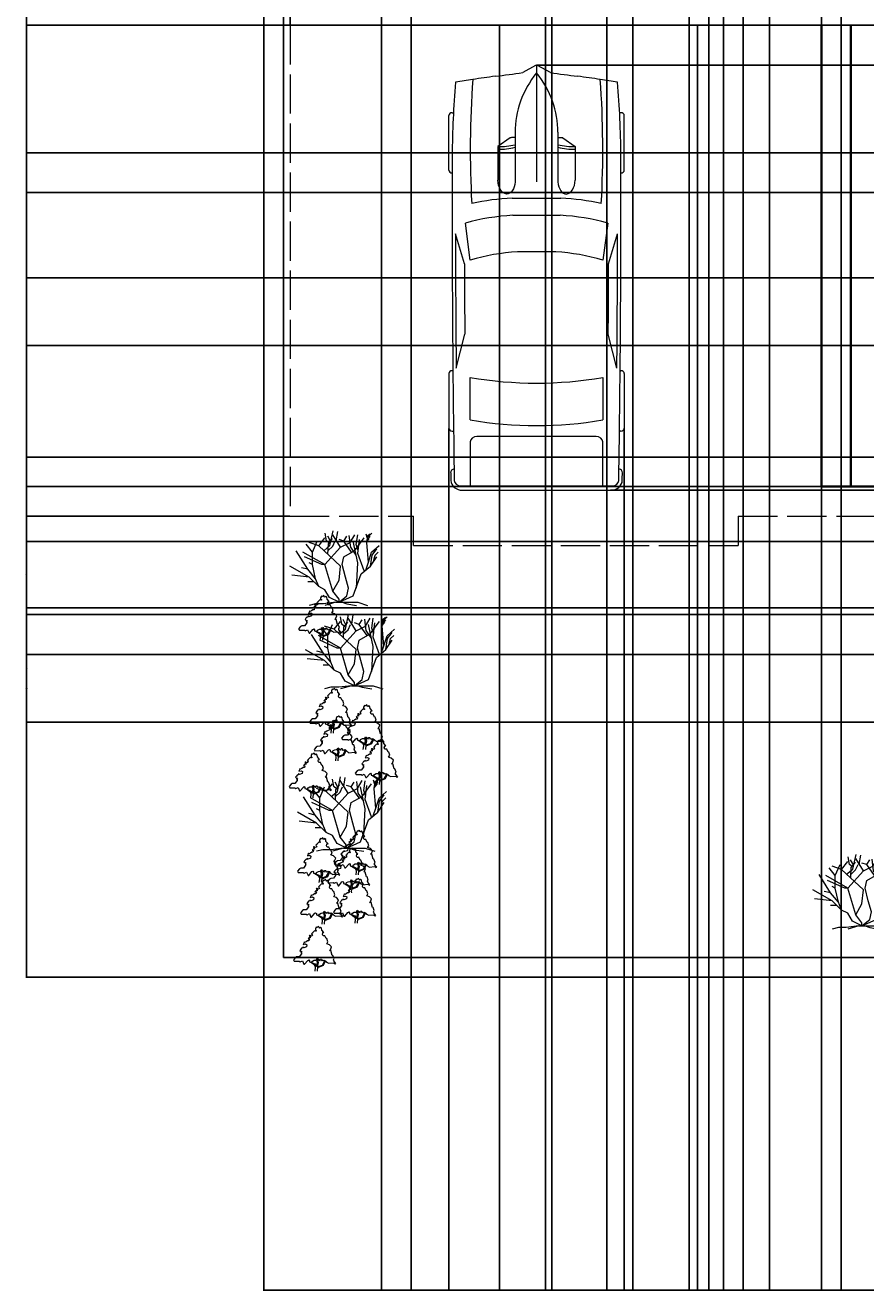
# Model space of a CAD drawing. Units: inches. Extents: x -47 to 496, y -43 to 706.
# Tile 1 of 6: x -47 to 209, y -43 to 344. Entities that reach past the tile are written whole.
import ezdxf

# ---------------------------------------------------------------- set-up
doc = ezdxf.new("R2010")
doc.units = ezdxf.units.IN
doc.linetypes.add('ACAD_ISO02W100', pattern=[15, 12, -3])
for name, color, linetype, lineweight in [('A-ANNO-DIMS', 2, 'Continuous', 18), ('A-ROOF-OVHD', 8, 'ACAD_ISO02W100', 18), ('C-PKNG-VEHI', 8, 'Continuous', 13), ('C-PROP', 7, 'Continuous', 25), ('L-PLNT', 3, 'Continuous', 13), ('WALL', 7, 'Continuous', 35)]:
    doc.layers.add(name, color=color, linetype=linetype, lineweight=lineweight)
doc.styles.get("Standard").update_dxf_attribs({"font": 'arial.ttf'})
doc.dimstyles.get("Standard").update_dxf_attribs({"dimtxt": 0.18, "dimasz": 0.18, "dimexe": 0.18, "dimexo": 0.0625, "dimgap": 0.09, "dimtad": 0, "dimtih": 1, "dimtoh": 1, "dimdec": 4, "dimzin": 0, "dimdsep": 46, "dimtxsty": 'Standard', "dimcen": 0.09, "dimadec": 0, "dimazin": 0, "dimtfac": 1, "dimtdec": 4, "dimtofl": 0, "dimtmove": 0, "dimatfit": 3, "dimfxl": 1, "dimtolj": 1, "dimtzin": 0, "dimarcsym": 0})

# ---------------------------------------------------------------- blocks, each defined once
blk = doc.blocks.new('*U3')
for p, q in [((21.1, 37.41), (21.1, 36.83)), ((46.55, 38.89), (22.35, 38.89)), ((47.8, 37.39), (47.8, 37.41)), ((87.99, 31.87), (74.76, 35.92)), ((134.31, 35.6), (119.29, 31.78)), ((135.45, 37.07), (135.45, 37.41)), ((136.7, 38.89), (160.9, 38.89)), ((162.15, 37.41), (162.15, 36.77)), ((70.03, 31.54), (86.41, 29.35)), ((138.42, 29.35), (157.25, 29.35)), ((186.47, 29.35), (167.01, 29.35)), ((186.47, -33.5), (186.47, 33.5)), ((188.4, -32.76), (188.4, 32.76)), ((164.52, 26.39), (164.52, -26.39)), ((32.27, 11.63), (36.13, 17.17)), ((36.13, 17.17), (50.94, 17.17)), ((3.27, 6.13), (0.1, 0.41)), ((29.77, 9.51), (51.68, 9.51)), ((32.12, 9.51), (32.12, 11.15)), ((58.92, -10.77), (58.92, 10.77)), ((66.55, -10.53), (66.55, 10.53)), ((82.74, 8.5), (82.74, -8.5)), ((186.47, -10.53), (186.47, 10.53)), ((0, 0), (51.68, 0)), ((0.1, -0.41), (3.27, -6.13)), ((29.77, -9.51), (51.68, -9.51)), ((32.12, -9.51), (32.12, -11.15)), ((32.27, -11.63), (36.13, -17.17)), ((36.13, -17.17), (50.94, -17.17)), ((86.41, -29.35), (70.03, -31.54)), ((87.99, -31.87), (74.76, -35.92)), ((134.31, -35.6), (119.29, -31.78)), ((157.25, -29.35), (138.42, -29.35)), ((167.01, -29.35), (186.47, -29.35)), ((21.1, -37.41), (21.1, -36.83)), ((46.55, -38.89), (22.35, -38.89)), ((47.8, -37.39), (47.8, -37.41)), ((135.45, -37.07), (135.45, -37.41)), ((136.7, -38.89), (160.9, -38.89)), ((162.15, -37.41), (162.15, -36.77))]:
    blk.add_line(p, q)
for centre, major_axis, ratio, start_param, end_param in [((266.03, -27.52), (0, 313.31), 0.842304, 1.367076, 1.39176), ((41.19, -490.86), (0, 528.23), 0.842304, 0.00281, 0.075598), ((22.35, 37.41), (0, -1.48), 0.842304, 3.141593, 4.712389), ((64.48, -10555.62), (0, 10593.03), 0.842304, -0.013397, 0.002797), ((46.55, 37.41), (0, 1.48), 0.842304, -1.570796, 0), ((64.48, -10555.62), (0, -10591.55), 0.842304, 3.133765, 3.140441), ((136.7, 37.41), (0, -1.48), 0.842304, 3.141593, 4.712389), ((160.9, 37.41), (0, 1.48), 0.842304, -1.570796, 0), ((180.63, 35.84), (0, 2.22), 0.842304, -0.013017, 1.249894), ((64.48, -10556.36), (0, 10595.31), 0.842304, -0.013397, -0.013017), ((183.98, 33.5), (0, -2.96), 0.842304, 1.570796, 3.128196), ((183.98, 32.76), (0, -5.25), 0.842304, 1.570796, 3.128196), ((259.18, -27.52), (0, -305.3), 0.842304, 4.528606, 4.561838), ((37.47, -593.96), (0, -623.33), 0.842304, 3.096046, 3.200911), ((134.4, 5.39), (0, -89.78), 0.842304, 4.449482, 4.652344), ((135.29, 5.39), (0, 81.77), 0.842304, 1.245306, 1.50788), ((149.6, 2.8), (0, -79.58), 0.842304, 4.372215, 4.640744), ((95.79, -3666.35), (0, -3698.24), 0.842304, 3.134049, 3.144098), ((17.08, 0), (0, 147.02), 0.842304, 4.511394, 4.913384), ((35.91, 0), (0, 147.02), 0.842304, 4.511394, 4.913384), ((167.01, 26.39), (0, 2.96), 0.842304, 0, 1.570796), ((-204.49, 52.4), (0, -250.96), 0.842304, 1.385369, 1.434372), ((13.04, 17.01), (0, 27.42), 0.842304, 4.435146, 4.718221), ((14.2, 17.01), (0, 27.42), 0.842304, 4.435146, 4.718221), ((50.79, 13.34), (6.34, -0.36), 0.603834, -1.395552, 1.581315), ((32.75, 11.15), (0, 0.74), 0.842304, 0.879714, 1.570796), ((29.77, -46.66), (0, 56.17), 0.842304, 0, 0.590319), ((0.62, 0), (0, -0.74), 0.842304, 4.131459, 5.293319), ((29.77, 46.66), (0, 56.17), 0.842304, 2.551274, 3.141593), ((-204.49, -52.4), (0, 250.96), 0.842304, -1.434372, -1.385369), ((32.75, -11.15), (0, -0.74), 0.842304, 4.712389, 5.403472), ((13.04, -17.01), (0, -27.42), 0.842304, 1.564964, 1.848039), ((14.2, -17.01), (0, -27.42), 0.842304, 1.564964, 1.848039), ((134.4, -5.39), (0, -89.78), 0.842304, -1.510751, -1.307889), ((135.29, -5.39), (0, -81.77), 0.842304, -1.50788, -1.245306), ((149.6, -2.8), (0, -79.58), 0.842304, -1.499151, -1.230623), ((259.18, 27.52), (0, 305.3), 0.842304, 1.721348, 1.754579), ((167.01, -26.39), (0, -2.96), 0.842304, 4.712389, 6.283185), ((266.03, 27.52), (0, 313.31), 0.842304, 1.749832, 1.774517), ((37.47, 593.96), (0, -623.33), 0.842304, -0.059319, 0.045547), ((95.79, 3666.35), (0, -3698.24), 0.842304, -0.002505, 0.007544), ((183.98, -33.5), (0, 2.96), 0.842304, 3.15499, 4.712389), ((183.98, -32.76), (0, -5.25), 0.842304, 0.013397, 1.570796), ((41.19, 490.86), (0, -528.23), 0.842304, -0.075598, -0.00281), ((22.35, -37.41), (0, 1.48), 0.842304, 1.570796, 3.141593), ((64.48, 10555.62), (0, 10593.03), 0.842304, 3.138796, 3.15499), ((46.55, -37.41), (0, -1.48), 0.842304, 0, 1.570796), ((64.48, 10555.62), (0, -10591.55), 0.842304, 0.001152, 0.007828), ((136.7, -37.41), (0, -1.48), 0.842304, -1.570796, 0), ((160.9, -37.41), (0, 1.48), 0.842304, 3.141593, 4.712389), ((180.63, -35.84), (0, -2.22), 0.842304, -1.249894, 0.013017), ((64.48, 10556.36), (0, 10595.31), 0.842304, 3.15461, 3.15499)]:
    blk.add_ellipse(centre, major_axis=major_axis, ratio=ratio, start_param=start_param, end_param=end_param)
at = {"extrusion": (0, 0, -1)}
blk.add_ellipse((50.79, -13.34), major_axis=(6.34, 0.36), ratio=0.603834, start_param=-1.395552, end_param=1.581315, dxfattribs=at)
blk = doc.blocks.new('*U6')
for p, q in [((-16.8, 16.32), (-15.36, 19.68)), ((-14.88, 18.24), (-12.96, 20.64)), ((-12.471, 19.775), (-12.898, 22.044)), ((-11.677, 19.071), (-12.471, 19.775)), ((-11.28, 19.619), (-12.104, 21.184)), ((-11.921, 18.836), (-10.64, 20.401)), ((-11.433, 18.289), (-10.457, 22.749)), ((-10.579, 18.054), (-9.846, 19.697)), ((-8.16, 17.76), (-10.56, 21.6)), ((-9.48, 19.775), (-8.992, 22.592)), ((-7.2, 19.68), (-8.64, 20.16)), ((-7.2, 19.68), (-6.24, 21.12)), ((-4.8, 16.32), (-7.2, 19.68)), ((-5.086, 17.741), (-5.513, 21.34)), ((-5.28, 19.2), (-3.84, 21.6)), ((-2.88, 12.96), (-4.32, 19.68)), ((-3.84, 16.8), (-0.96, 20.64)), ((-3.377, 18.602), (-2.888, 21.575)), ((-2.88, 15.84), (-2.4, 20.16)), ((-0.508, 21.888), (-0.081, 20.558)), ((-0.203, 19.149), (0.102, 21.34)), ((-0.142, 19.384), (0.59, 20.401)), ((-0.02, 20.01), (0.896, 21.105)), ((0.041, 20.714), (1.384, 22.044)), ((0.102, 21.34), (0.835, 21.888)), ((-18.24, 11.04), (-21.755, 16.655)), ((-12.96, 12.48), (-19.68, 16.32)), ((-16.8, 16.32), (-18.72, 18.72)), ((-14.88, 18.24), (-17.76, 19.2)), ((-16.8, 12.48), (-16.8, 16.32)), ((-8.16, 12), (-14.88, 18.24)), ((-13.325, 16.724), (-11.433, 18.289)), ((-12.96, 12.48), (-8.16, 17.76)), ((-12.043, 15.628), (-11.921, 18.836)), ((-11.982, 16.802), (-10.579, 18.054)), ((-8.16, 17.76), (-5.28, 19.2)), ((-7.2, 14.88), (-3.84, 16.8)), ((-3.377, 15.315), (-5.086, 17.819)), ((-2.766, 16.802), (-3.377, 18.602)), ((-0.96, 10.56), (-2.88, 15.84)), ((0.346, 13.203), (-0.203, 19.149)), ((0.346, 13.203), (1.323, 16.254)), ((1.323, 16.254), (3.642, 18.289)), ((1.44, 15.36), (2.88, 17.28)), ((2.4, 15.36), (3.36, 16.32)), ((-17.76, 8.64), (-23.663, 11.961)), ((-13.92, 12.48), (-19.2, 14.88)), ((-16.8, 12.48), (-17.76, 12.96)), ((-15.84, 8.16), (-16.8, 12.48)), ((-12.96, 12.48), (-13.92, 12.48)), ((-10.56, 4.32), (-12.96, 12.48)), ((-8.64, 7.68), (-8.16, 12)), ((-7.68, 12.48), (-7.2, 14.88)), ((-6.72, 8.64), (-7.68, 12.48)), ((-3.36, 5.28), (-2.88, 12.96)), ((-1.92, 9.6), (0.96, 12)), ((-0.48, 10.8), (0.346, 13.203)), ((0.96, 12), (1.44, 15.36)), ((0.96, 12), (2.88, 14.88)), ((1.92, 13.44), (2.4, 15.36)), ((-17.76, 8.64), (-23.128, 9.222)), ((-18.24, 11.04), (-20.16, 11.52)), ((-15.84, 8.16), (-18.24, 11.04)), ((-14.88, 5.76), (-17.76, 8.64)), ((-14.88, 5.76), (-15.84, 8.16)), ((-5.76, 5.28), (-6.72, 8.64)), ((-4.32, 2.88), (-1.92, 9.6)), ((-16.32, 7.2), (-18.24, 7.2)), ((-12.96, 4.8), (-14.88, 5.76)), ((-11.52, 2.4), (-12.96, 4.8)), ((-10.56, 4.32), (-8.64, 7.68)), ((-8.64, 1.92), (-10.56, 4.32)), ((-6.24, 2.88), (-5.76, 5.28)), ((-15.84, 0.48), (-17.76, 0)), ((-13.44, 0.48), (-15.84, 0.48)), ((-9.6, 0.96), (-13.44, 0.48)), ((-9.6, 0.96), (-12.96, 0)), ((-8.64, 0.96), (-11.52, 2.4)), ((-9.6, 0.96), (-7.68, 0.96)), ((-8.64, 0.96), (-4.32, 2.88)), ((-8.64, 0.96), (-6.24, 2.88)), ((-8.64, 0.96), (-8.64, 1.92)), ((-8.64, 0.96), (-2.88, 0.96)), ((-7.68, 0.96), (-6.24, 0.48)), ((-6.24, 0.48), (-3.36, 0)), ((-2.88, 0.96), (0, 0))]:
    blk.add_line(p, q)
blk = doc.blocks.new('*U7')
for points in [[(22.0124, 137.721), (18.5475, 141.5624), (15.5282, 138.2446), (13.8028, 139.3505), (13.3714, 142.1153), (11.2148, 143.2214), (8.1954, 140.4564), (4.7447, 141.0094), (2.1567, 136.0326), (2.1567, 131.6088), (5.6074, 129.9499), (3.0193, 128.2909), (0.4313, 130.5029), (-6.9015, 123.3141), (-6.9015, 121.6552), (-9.9208, 119.9963), (-9.0581, 118.3373), (-6.9015, 115.0195), (-10.7835, 112.2546), (-14.6656, 115.0195), (-16.8222, 114.4665), (-17.6849, 112.2546), (-14.6656, 111.7016), (-14.2342, 107.2778), (-17.6065, 107.8307), (-21.5669, 103.9599), (-17.2536, 103.4069), (-18.9789, 97.8771), (-22.8609, 97.3241), (-27.1743, 94.5593), (-32.3504, 91.7944), (-32.7817, 94.0063), (-36.6638, 85.7116), (-29.7624, 87.3705), (-25.449, 84.6056), (-26.743, 77.9699), (-34.507, 75.205), (-37.9578, 77.4169), (-39.2518, 74.099), (-42.2711, 73.5461), (-44.8592, 70.2282), (-47.8786, 66.3574), (-43.9965, 63.0395), (-41.4085, 64.6985), (-44.3346, 59.8898), (-42.2089, 60.1377), (-42.5159, 55.7849), (-49.6039, 46.4502), (-58.2307, 45.8972), (-62.1127, 43.6853), (-68.5828, 36.4966), (-65.9947, 32.0727), (-50.0352, 32.6257), (-47.0159, 30.4138), (-39.6831, 33.7317), (-34.507, 22.6721), (-32.3504, 22.6721), (-22.4296, 34.8376), (-19.4102, 36.4966), (-17.2536, 33.7317), (-17.2536, 29.8608), (-13.8028, 28.7549), (-9.0581, 28.7549), (-7.3328, 32.6257), (-1.7254, 35.3906), (3.8821, 35.9436), (6.4701, 38.1555), (6.9014, 38.7085), (8.1954, 41.4734), (9.9208, 40.3674), (11.2148, 35.9436), (14.2341, 37.6025), (15.0968, 36.4966), (15.9595, 33.7317), (18.9789, 38.7085), (21.9982, 38.7085), (23.2922, 36.4966), (21.9982, 34.2847), (25.4489, 35.3906), (26.743, 33.7317), (29.7623, 35.9436), (32.7817, 34.8376), (38.8204, 28.7549), (41.4084, 27.6489), (43.5651, 25.437), (61.6813, 27.0959), (65.132, 23.7781), (67.7201, 24.884), (60.8186, 33.7317), (60.3873, 37.0495), (62.544, 40.3674), (58.662, 50.874), (56.5053, 50.874), (52.1919, 66.3574), (47.8785, 66.9103), (50.4665, 69.1222), (53.9172, 77.9699), (47.0158, 85.1586), (38.3891, 87.9235), (42.2711, 94.0063)], [(42.2711, 94.0063), (38.8204, 104.5129), (36.6637, 104.5129), (32.3503, 113.9135), (29.7623, 113.3605), (26.743, 113.3605), (24.5862, 117.7844), (25.8802, 123.8671), (29.331, 123.8671), (22.8609, 131.6088), (21.9982, 137.6916)], [(-12.9401, 28.7549), (-2.588, 22.1191), (0.8626, 17.6953), (1.7253, 11.6125), (0, 0)], [(-9.9208, 28.2019), (0, 23.2251), (3.4507, 19.9072), (4.7447, 15.4834), (8.6267, 27.0959), (6.4701, 37.6025)], [(34.5071, 33.1787), (27.1743, 18.2483), (9.0581, 10.5066), (7.7641, 3.8708), (8.1954, 0)], [(8.1954, 40.3674), (11.2148, 27.6489), (8.1954, 13.8245), (24.5862, 19.9072), (32.7817, 34.2847)]]:
    blk.add_lwpolyline(points)
blk = doc.blocks.new('*D12')
at = {"layer": 'A-ANNO-DIMS', "color": 0, "lineweight": -2, "transparency": 16777216}
for p, q in [((25.45, 52.91), (25.45, -42.84)), ((395.45, 52.91), (395.45, -42.84)), ((25.63, -42.66), (210.17, -42.66)), ((395.27, -42.66), (210.74, -42.66))]:
    blk.add_line(p, q, dxfattribs=at)
at = {"layer": 'A-ANNO-DIMS', "color": 0, "transparency": 16777216}
for points in [[(25.63, -42.63), (25.63, -42.69), (25.45, -42.66)], [(395.27, -42.63), (395.27, -42.69), (395.45, -42.66)]]:
    blk.add_solid(points, dxfattribs=at)
at = {"layer": 'Defpoints', "color": 0, "transparency": 16777216}
for p in [(25.45, 52.97), (395.45, 52.97), (395.45, -42.66)]:
    blk.add_point(p, dxfattribs=at)
at = {"layer": 'A-ANNO-DIMS', "color": 0, "transparency": 16777216, "insert": (210.45, -42.66), "char_height": 0.18, "attachment_point": 5}
blk.add_mtext('\\A1;370', dxfattribs=at)
blk = doc.blocks.new('*D13')
at = {"layer": 'A-ANNO-DIMS', "color": 0, "lineweight": -2, "transparency": 16777216}
for p, q in [((25.39, 671.47), (-47.29, 671.47)), ((-47.11, 671.29), (-47.11, 362.4)), ((-47.11, 53.15), (-47.11, 362.04)), ((25.39, 52.97), (-47.29, 52.97))]:
    blk.add_line(p, q, dxfattribs=at)
at = {"layer": 'A-ANNO-DIMS', "color": 0, "transparency": 16777216}
for points in [[(-47.14, 671.29), (-47.08, 671.29), (-47.11, 671.47)], [(-47.14, 53.15), (-47.08, 53.15), (-47.11, 52.97)]]:
    blk.add_solid(points, dxfattribs=at)
at = {"layer": 'Defpoints', "color": 0, "transparency": 16777216}
for p in [(-47.11, 671.47), (25.45, 671.47), (25.45, 52.97)]:
    blk.add_point(p, dxfattribs=at)
at = {"layer": 'A-ANNO-DIMS', "color": 0, "transparency": 16777216, "insert": (-47.11, 362.22), "char_height": 0.18, "attachment_point": 5}
blk.add_mtext('\\A1;618.5', dxfattribs=at)
blk = doc.blocks.new('*D25')
at = {"layer": 'A-ANNO-DIMS', "color": 0, "lineweight": -2, "transparency": 16777216}
for p, q in [((314.47, 186.18), (-47.29, 186.18)), ((-47.11, 186), (-47.11, 176.21)), ((-47.11, 166.05), (-47.11, 175.84)), ((314.47, 165.87), (-47.29, 165.87))]:
    blk.add_line(p, q, dxfattribs=at)
at = {"layer": 'A-ANNO-DIMS', "color": 0, "transparency": 16777216}
for points in [[(-47.14, 186), (-47.08, 186), (-47.11, 186.18)], [(-47.14, 166.05), (-47.08, 166.05), (-47.11, 165.87)]]:
    blk.add_solid(points, dxfattribs=at)
at = {"layer": 'Defpoints', "color": 0, "transparency": 16777216}
for p in [(-47.11, 186.18), (314.53, 186.18), (314.53, 165.87)]:
    blk.add_point(p, dxfattribs=at)
at = {"layer": 'A-ANNO-DIMS', "color": 0, "transparency": 16777216, "insert": (-47.11, 176.03), "char_height": 0.18, "attachment_point": 5}
blk.add_mtext('\\A1;20.318', dxfattribs=at)
blk = doc.blocks.new('*D27')
at = {"layer": 'A-ANNO-DIMS', "color": 0, "lineweight": -2, "transparency": 16777216}
for p, q in [((229.82, 163.83), (-47.29, 163.83)), ((-47.11, 163.65), (-47.11, 147.58)), ((-47.11, 131.15), (-47.11, 147.22)), ((213.89, 130.97), (-47.29, 130.97))]:
    blk.add_line(p, q, dxfattribs=at)
at = {"layer": 'A-ANNO-DIMS', "color": 0, "transparency": 16777216}
for points in [[(-47.14, 163.65), (-47.08, 163.65), (-47.11, 163.83)], [(-47.14, 131.15), (-47.08, 131.15), (-47.11, 130.97)]]:
    blk.add_solid(points, dxfattribs=at)
at = {"layer": 'Defpoints', "color": 0, "transparency": 16777216}
for p in [(-47.11, 163.83), (229.88, 163.83), (213.95, 130.97)]:
    blk.add_point(p, dxfattribs=at)
at = {"layer": 'A-ANNO-DIMS', "color": 0, "transparency": 16777216, "insert": (-47.11, 147.4), "char_height": 0.18, "attachment_point": 5}
blk.add_mtext('\\A1;32.864', dxfattribs=at)
blk = doc.blocks.new('*D31')
at = {"layer": 'A-ANNO-DIMS', "color": 0, "lineweight": -2, "transparency": 16777216}
for p, q in [((285.55, 151.67), (-47.29, 151.67)), ((-47.11, 151.49), (-47.11, 141.5)), ((-47.11, 131.15), (-47.11, 141.14)), ((359.39, 130.97), (-47.29, 130.97))]:
    blk.add_line(p, q, dxfattribs=at)
at = {"layer": 'A-ANNO-DIMS', "color": 0, "transparency": 16777216}
for points in [[(-47.14, 151.49), (-47.08, 151.49), (-47.11, 151.67)], [(-47.14, 131.15), (-47.08, 131.15), (-47.11, 130.97)]]:
    blk.add_solid(points, dxfattribs=at)
at = {"layer": 'Defpoints', "color": 0, "transparency": 16777216}
for p in [(285.61, 151.67), (-47.11, 130.97), (359.45, 130.97)]:
    blk.add_point(p, dxfattribs=at)
at = {"layer": 'A-ANNO-DIMS', "color": 0, "transparency": 16777216, "insert": (-47.11, 141.32), "char_height": 0.18, "attachment_point": 5}
blk.add_mtext('\\A1;20.695', dxfattribs=at)
blk = doc.blocks.new('*D41')
at = {"layer": 'A-ANNO-DIMS', "color": 0, "lineweight": -2, "transparency": 16777216}
for p, q in [((111.58, 621.91), (111.58, -42.84)), ((138.26, 621.91), (138.26, -42.84)), ((111.76, -42.66), (124.45, -42.66)), ((138.08, -42.66), (125.38, -42.66))]:
    blk.add_line(p, q, dxfattribs=at)
at = {"layer": 'A-ANNO-DIMS', "color": 0, "transparency": 16777216}
for points in [[(111.76, -42.63), (111.76, -42.69), (111.58, -42.66)], [(138.08, -42.63), (138.08, -42.69), (138.26, -42.66)]]:
    blk.add_solid(points, dxfattribs=at)
at = {"layer": 'Defpoints', "color": 0, "transparency": 16777216}
for p in [(111.58, 621.97), (138.26, 621.97), (138.26, -42.66)]:
    blk.add_point(p, dxfattribs=at)
at = {"layer": 'A-ANNO-DIMS', "color": 0, "transparency": 16777216, "insert": (124.92, -42.66), "char_height": 0.18, "attachment_point": 5}
blk.add_mtext('\\A1;26.675', dxfattribs=at)
blk = doc.blocks.new('*D42')
at = {"layer": 'A-ANNO-DIMS', "color": 0, "lineweight": -2, "transparency": 16777216}
for p, q in [((70.45, 621.91), (70.45, -42.84)), ((111.58, 621.91), (111.58, -42.84)), ((70.63, -42.66), (90.55, -42.66)), ((111.4, -42.66), (91.48, -42.66))]:
    blk.add_line(p, q, dxfattribs=at)
at = {"layer": 'A-ANNO-DIMS', "color": 0, "transparency": 16777216}
for points in [[(70.63, -42.63), (70.63, -42.69), (70.45, -42.66)], [(111.4, -42.63), (111.4, -42.69), (111.58, -42.66)]]:
    blk.add_solid(points, dxfattribs=at)
at = {"layer": 'Defpoints', "color": 0, "transparency": 16777216}
for p in [(70.45, 621.97), (111.58, 621.97), (111.58, -42.66)]:
    blk.add_point(p, dxfattribs=at)
at = {"layer": 'A-ANNO-DIMS', "color": 0, "transparency": 16777216, "insert": (91.02, -42.66), "char_height": 0.18, "attachment_point": 5}
blk.add_mtext('\\A1;41.125', dxfattribs=at)
blk = doc.blocks.new('*D45')
at = {"layer": 'A-ANNO-DIMS', "color": 0, "lineweight": -2, "transparency": 16777216}
for p, q in [((113.45, 480.41), (113.45, -42.84)), ((155.45, 480.41), (155.45, -42.84)), ((113.63, -42.66), (134.23, -42.66)), ((155.27, -42.66), (134.68, -42.66))]:
    blk.add_line(p, q, dxfattribs=at)
at = {"layer": 'A-ANNO-DIMS', "color": 0, "transparency": 16777216}
for points in [[(113.63, -42.63), (113.63, -42.69), (113.45, -42.66)], [(155.27, -42.63), (155.27, -42.69), (155.45, -42.66)]]:
    blk.add_solid(points, dxfattribs=at)
at = {"layer": 'Defpoints', "color": 0, "transparency": 16777216}
for p in [(113.45, 480.47), (155.45, 480.47), (155.45, -42.66)]:
    blk.add_point(p, dxfattribs=at)
at = {"layer": 'A-ANNO-DIMS', "color": 0, "transparency": 16777216, "insert": (134.45, -42.66), "char_height": 0.18, "attachment_point": 5}
blk.add_mtext('\\A1;42', dxfattribs=at)
blk = doc.blocks.new('*D46')
at = {"layer": 'A-ANNO-DIMS', "color": 0, "lineweight": -2, "transparency": 16777216}
for p, q in [((70.45, 480.41), (70.45, -42.84)), ((113.45, 480.41), (113.45, -42.84)), ((70.63, -42.66), (91.73, -42.66)), ((113.27, -42.66), (92.18, -42.66))]:
    blk.add_line(p, q, dxfattribs=at)
at = {"layer": 'A-ANNO-DIMS', "color": 0, "transparency": 16777216}
for points in [[(70.63, -42.63), (70.63, -42.69), (70.45, -42.66)], [(113.27, -42.63), (113.27, -42.69), (113.45, -42.66)]]:
    blk.add_solid(points, dxfattribs=at)
at = {"layer": 'Defpoints', "color": 0, "transparency": 16777216}
for p in [(70.45, 480.47), (113.45, 480.47), (113.45, -42.66)]:
    blk.add_point(p, dxfattribs=at)
at = {"layer": 'A-ANNO-DIMS', "color": 0, "transparency": 16777216, "insert": (91.95, -42.66), "char_height": 0.18, "attachment_point": 5}
blk.add_mtext('\\A1;43', dxfattribs=at)
blk = doc.blocks.new('*D47')
at = {"layer": 'A-ANNO-DIMS', "color": 0, "lineweight": -2, "transparency": 16777216}
for p, q in [((171.95, 480.41), (171.95, -42.84)), ((201.95, 480.41), (201.95, -42.84)), ((172.13, -42.66), (186.74, -42.66)), ((201.77, -42.66), (187.17, -42.66))]:
    blk.add_line(p, q, dxfattribs=at)
at = {"layer": 'A-ANNO-DIMS', "color": 0, "transparency": 16777216}
for points in [[(172.13, -42.63), (172.13, -42.69), (171.95, -42.66)], [(201.77, -42.63), (201.77, -42.69), (201.95, -42.66)]]:
    blk.add_solid(points, dxfattribs=at)
at = {"layer": 'Defpoints', "color": 0, "transparency": 16777216}
for p in [(171.95, 480.47), (201.95, 480.47), (201.95, -42.66)]:
    blk.add_point(p, dxfattribs=at)
at = {"layer": 'A-ANNO-DIMS', "color": 0, "transparency": 16777216, "insert": (186.95, -42.66), "char_height": 0.18, "attachment_point": 5}
blk.add_mtext('\\A1;30', dxfattribs=at)
blk = doc.blocks.new('*D49')
at = {"layer": 'A-ANNO-DIMS', "color": 0, "lineweight": -2, "transparency": 16777216}
for p, q in [((61.45, 635.41), (61.45, -42.84)), ((70.45, 635.41), (70.45, -42.84)), ((61.63, -42.66), (65.81, -42.66)), ((70.27, -42.66), (66.1, -42.66))]:
    blk.add_line(p, q, dxfattribs=at)
at = {"layer": 'A-ANNO-DIMS', "color": 0, "transparency": 16777216}
for points in [[(61.63, -42.63), (61.63, -42.69), (61.45, -42.66)], [(70.27, -42.63), (70.27, -42.69), (70.45, -42.66)]]:
    blk.add_solid(points, dxfattribs=at)
at = {"layer": 'Defpoints', "color": 0, "transparency": 16777216}
for p in [(61.45, 635.47), (70.45, 635.47), (70.45, -42.66)]:
    blk.add_point(p, dxfattribs=at)
at = {"layer": 'A-ANNO-DIMS', "color": 0, "transparency": 16777216, "insert": (65.95, -42.66), "char_height": 0.18, "attachment_point": 5}
blk.add_mtext('\\A1;9', dxfattribs=at)
blk = doc.blocks.new('*D50')
at = {"layer": 'A-ANNO-DIMS', "color": 0, "lineweight": -2, "transparency": 16777216}
for p, q in [((161.45, 621.91), (161.45, -42.84)), ((165.95, 621.91), (165.95, -42.84)), ((161.63, -42.66), (163.45, -42.66)), ((165.77, -42.66), (163.96, -42.66))]:
    blk.add_line(p, q, dxfattribs=at)
at = {"layer": 'A-ANNO-DIMS', "color": 0, "transparency": 16777216}
for points in [[(161.63, -42.63), (161.63, -42.69), (161.45, -42.66)], [(165.77, -42.63), (165.77, -42.69), (165.95, -42.66)]]:
    blk.add_solid(points, dxfattribs=at)
at = {"layer": 'Defpoints', "color": 0, "transparency": 16777216}
for p in [(161.45, 621.97), (165.95, 621.97), (165.95, -42.66)]:
    blk.add_point(p, dxfattribs=at)
at = {"layer": 'A-ANNO-DIMS', "color": 0, "transparency": 16777216, "insert": (163.7, -42.66), "char_height": 0.18, "attachment_point": 5}
blk.add_mtext('\\A1;4.5', dxfattribs=at)
blk = doc.blocks.new('*D62')
at = {"layer": 'A-ANNO-DIMS', "color": 0, "lineweight": -2, "transparency": 16777216}
for p, q in [((70.45, 348.41), (70.45, -42.84)), ((97.54, 343.91), (97.54, -42.84)), ((70.63, -42.66), (83.6, -42.66)), ((97.36, -42.66), (84.39, -42.66))]:
    blk.add_line(p, q, dxfattribs=at)
at = {"layer": 'A-ANNO-DIMS', "color": 0, "transparency": 16777216}
for points in [[(70.63, -42.63), (70.63, -42.69), (70.45, -42.66)], [(97.36, -42.63), (97.36, -42.69), (97.54, -42.66)]]:
    blk.add_solid(points, dxfattribs=at)
at = {"layer": 'Defpoints', "color": 0, "transparency": 16777216}
for p in [(70.45, 348.47), (97.54, 343.97), (97.54, -42.66)]:
    blk.add_point(p, dxfattribs=at)
at = {"layer": 'A-ANNO-DIMS', "color": 0, "transparency": 16777216, "insert": (84, -42.66), "char_height": 0.18, "attachment_point": 5}
blk.add_mtext('\\A1;27.09', dxfattribs=at)
blk = doc.blocks.new('*D63')
at = {"layer": 'A-ANNO-DIMS', "color": 0, "lineweight": -2, "transparency": 16777216}
for p, q in [((97.54, 343.91), (97.54, -42.84)), ((158.02, 343.91), (158.02, -42.84)), ((97.72, -42.66), (127.39, -42.66)), ((157.84, -42.66), (128.18, -42.66))]:
    blk.add_line(p, q, dxfattribs=at)
at = {"layer": 'A-ANNO-DIMS', "color": 0, "transparency": 16777216}
for points in [[(97.72, -42.63), (97.72, -42.69), (97.54, -42.66)], [(157.84, -42.63), (157.84, -42.69), (158.02, -42.66)]]:
    blk.add_solid(points, dxfattribs=at)
at = {"layer": 'Defpoints', "color": 0, "transparency": 16777216}
for p in [(97.54, 343.97), (158.02, 343.97), (158.02, -42.66)]:
    blk.add_point(p, dxfattribs=at)
at = {"layer": 'A-ANNO-DIMS', "color": 0, "transparency": 16777216, "insert": (127.78, -42.66), "char_height": 0.18, "attachment_point": 5}
blk.add_mtext('\\A1;60.48', dxfattribs=at)
blk = doc.blocks.new('*D64')
at = {"layer": 'A-ANNO-DIMS', "color": 0, "lineweight": -2, "transparency": 16777216}
for p, q in [((158.02, 343.91), (158.02, -42.84)), ((218.45, 343.91), (218.45, -42.84)), ((158.2, -42.66), (187.84, -42.66)), ((218.27, -42.66), (188.63, -42.66))]:
    blk.add_line(p, q, dxfattribs=at)
at = {"layer": 'A-ANNO-DIMS', "color": 0, "transparency": 16777216}
for points in [[(158.2, -42.63), (158.2, -42.69), (158.02, -42.66)], [(218.27, -42.63), (218.27, -42.69), (218.45, -42.66)]]:
    blk.add_solid(points, dxfattribs=at)
at = {"layer": 'Defpoints', "color": 0, "transparency": 16777216}
for p in [(158.02, 343.97), (218.45, 343.97), (218.45, -42.66)]:
    blk.add_point(p, dxfattribs=at)
at = {"layer": 'A-ANNO-DIMS', "color": 0, "transparency": 16777216, "insert": (188.24, -42.66), "char_height": 0.18, "attachment_point": 5}
blk.add_mtext('\\A1;60.43', dxfattribs=at)
blk = doc.blocks.new('*D66')
at = {"layer": 'A-ANNO-DIMS', "color": 0, "lineweight": -2, "transparency": 16777216}
for p, q in [((130.34, 396.56), (130.34, -42.84)), ((180.05, 396.56), (180.05, -42.84)), ((130.52, -42.66), (154.82, -42.66)), ((179.87, -42.66), (155.58, -42.66))]:
    blk.add_line(p, q, dxfattribs=at)
at = {"layer": 'A-ANNO-DIMS', "color": 0, "transparency": 16777216}
for points in [[(130.52, -42.63), (130.52, -42.69), (130.34, -42.66)], [(179.87, -42.63), (179.87, -42.69), (180.05, -42.66)]]:
    blk.add_solid(points, dxfattribs=at)
at = {"layer": 'Defpoints', "color": 0, "transparency": 16777216}
for p in [(130.34, 396.63), (180.05, 396.63), (180.05, -42.66)]:
    blk.add_point(p, dxfattribs=at)
at = {"layer": 'A-ANNO-DIMS', "color": 0, "transparency": 16777216, "insert": (155.2, -42.66), "char_height": 0.18, "attachment_point": 5}
blk.add_mtext('\\A1;49.71', dxfattribs=at)
blk = doc.blocks.new('*D70')
at = {"layer": 'A-ANNO-DIMS', "color": 0, "lineweight": -2, "transparency": 16777216}
for p, q in [((33.45, 344.03), (33.45, 705.7)), ((33.63, 705.52), (114.32, 705.52)), ((195.77, 705.52), (115.09, 705.52)), ((195.95, 344.03), (195.95, 705.7))]:
    blk.add_line(p, q, dxfattribs=at)
at = {"layer": 'A-ANNO-DIMS', "color": 0, "transparency": 16777216}
for points in [[(33.63, 705.55), (33.63, 705.49), (33.45, 705.52)], [(195.77, 705.55), (195.77, 705.49), (195.95, 705.52)]]:
    blk.add_solid(points, dxfattribs=at)
at = {"layer": 'Defpoints', "color": 0, "transparency": 16777216}
for p in [(195.95, 705.52), (33.45, 343.97), (195.95, 343.97)]:
    blk.add_point(p, dxfattribs=at)
at = {"layer": 'A-ANNO-DIMS', "color": 0, "transparency": 16777216, "insert": (114.7, 705.52), "char_height": 0.18, "attachment_point": 5}
blk.add_mtext('\\A1;162.5', dxfattribs=at)
blk = doc.blocks.new('*D71')
at = {"layer": 'A-ANNO-DIMS', "color": 0, "lineweight": -2, "transparency": 16777216}
for p, q in [((33.39, 343.97), (-47.29, 343.97)), ((-47.11, 343.79), (-47.11, 269.15)), ((-47.11, 194.15), (-47.11, 268.79)), ((33.39, 193.97), (-47.29, 193.97))]:
    blk.add_line(p, q, dxfattribs=at)
at = {"layer": 'A-ANNO-DIMS', "color": 0, "transparency": 16777216}
for points in [[(-47.14, 343.79), (-47.08, 343.79), (-47.11, 343.97)], [(-47.14, 194.15), (-47.08, 194.15), (-47.11, 193.97)]]:
    blk.add_solid(points, dxfattribs=at)
at = {"layer": 'Defpoints', "color": 0, "transparency": 16777216}
for p in [(-47.11, 343.97), (33.45, 343.97), (33.45, 193.97)]:
    blk.add_point(p, dxfattribs=at)
at = {"layer": 'A-ANNO-DIMS', "color": 0, "transparency": 16777216, "insert": (-47.11, 268.97), "char_height": 0.18, "attachment_point": 5}
blk.add_mtext('\\A1;150', dxfattribs=at)
blk = doc.blocks.new('*D72')
at = {"layer": 'A-ANNO-DIMS', "color": 0, "lineweight": -2, "transparency": 16777216}
for p, q in [((195.89, 343.97), (-47.29, 343.97)), ((-47.11, 343.79), (-47.11, 273.65)), ((-47.11, 203.15), (-47.11, 273.29)), ((195.89, 202.97), (-47.29, 202.97))]:
    blk.add_line(p, q, dxfattribs=at)
at = {"layer": 'A-ANNO-DIMS', "color": 0, "transparency": 16777216}
for points in [[(-47.14, 343.79), (-47.08, 343.79), (-47.11, 343.97)], [(-47.14, 203.15), (-47.08, 203.15), (-47.11, 202.97)]]:
    blk.add_solid(points, dxfattribs=at)
at = {"layer": 'Defpoints', "color": 0, "transparency": 16777216}
for p in [(-47.11, 343.97), (195.95, 343.97), (195.95, 202.97)]:
    blk.add_point(p, dxfattribs=at)
at = {"layer": 'A-ANNO-DIMS', "color": 0, "transparency": 16777216, "insert": (-47.11, 273.47), "char_height": 0.18, "attachment_point": 5}
blk.add_mtext('\\A1;141', dxfattribs=at)
blk = doc.blocks.new('*D73')
at = {"layer": 'A-ANNO-DIMS', "color": 0, "lineweight": -2, "transparency": 16777216}
for p, q in [((213.95, 211.91), (213.95, -42.84)), ((195.95, 202.91), (195.95, -42.84)), ((196.13, -42.66), (204.74, -42.66)), ((213.77, -42.66), (205.17, -42.66))]:
    blk.add_line(p, q, dxfattribs=at)
at = {"layer": 'A-ANNO-DIMS', "color": 0, "transparency": 16777216}
for points in [[(196.13, -42.63), (196.13, -42.69), (195.95, -42.66)], [(213.77, -42.63), (213.77, -42.69), (213.95, -42.66)]]:
    blk.add_solid(points, dxfattribs=at)
at = {"layer": 'Defpoints', "color": 0, "transparency": 16777216}
for p in [(213.95, 211.97), (195.95, 202.97), (213.95, -42.66)]:
    blk.add_point(p, dxfattribs=at)
at = {"layer": 'A-ANNO-DIMS', "color": 0, "transparency": 16777216, "insert": (204.95, -42.66), "char_height": 0.18, "attachment_point": 5}
blk.add_mtext('\\A1;18', dxfattribs=at)
blk = doc.blocks.new('*D79')
at = {"layer": 'A-ANNO-DIMS', "color": 0, "lineweight": -2, "transparency": 16777216}
for p, q in [((311.88, 246.07), (-47.29, 246.07)), ((-47.11, 245.89), (-47.11, 229.2)), ((-47.11, 212.15), (-47.11, 228.84)), ((311.88, 211.97), (-47.29, 211.97))]:
    blk.add_line(p, q, dxfattribs=at)
at = {"layer": 'A-ANNO-DIMS', "color": 0, "transparency": 16777216}
for points in [[(-47.14, 245.89), (-47.08, 245.89), (-47.11, 246.07)], [(-47.14, 212.15), (-47.08, 212.15), (-47.11, 211.97)]]:
    blk.add_solid(points, dxfattribs=at)
at = {"layer": 'Defpoints', "color": 0, "transparency": 16777216}
for p in [(-47.11, 246.07), (311.95, 246.07), (311.95, 211.97)]:
    blk.add_point(p, dxfattribs=at)
at = {"layer": 'A-ANNO-DIMS', "color": 0, "transparency": 16777216, "insert": (-47.11, 229.02), "char_height": 0.18, "attachment_point": 5}
blk.add_mtext('\\A1;34.103', dxfattribs=at)
blk = doc.blocks.new('*D81')
at = {"layer": 'A-ANNO-DIMS', "color": 0, "lineweight": -2, "transparency": 16777216}
for p, q in [((213.89, 343.97), (-47.29, 343.97)), ((-47.11, 343.79), (-47.11, 318.58)), ((-47.11, 293.01), (-47.11, 318.22)), ((213.89, 292.83), (-47.29, 292.83))]:
    blk.add_line(p, q, dxfattribs=at)
at = {"layer": 'A-ANNO-DIMS', "color": 0, "transparency": 16777216}
for points in [[(-47.14, 343.79), (-47.08, 343.79), (-47.11, 343.97)], [(-47.14, 293.01), (-47.08, 293.01), (-47.11, 292.83)]]:
    blk.add_solid(points, dxfattribs=at)
at = {"layer": 'Defpoints', "color": 0, "transparency": 16777216}
for p in [(-47.11, 343.97), (213.95, 343.97), (213.95, 292.83)]:
    blk.add_point(p, dxfattribs=at)
at = {"layer": 'A-ANNO-DIMS', "color": 0, "transparency": 16777216, "insert": (-47.11, 318.4), "char_height": 0.18, "attachment_point": 5}
blk.add_mtext('\\A1;51.15', dxfattribs=at)
blk = doc.blocks.new('*D82')
at = {"layer": 'A-ANNO-DIMS', "color": 0, "lineweight": -2, "transparency": 16777216}
for p, q in [((108.88, 331.8), (496.14, 331.8)), ((495.96, 331.62), (495.96, 267)), ((495.96, 202.02), (495.96, 266.64)), ((131.48, 201.84), (496.14, 201.84))]:
    blk.add_line(p, q, dxfattribs=at)
at = {"layer": 'A-ANNO-DIMS', "color": 0, "transparency": 16777216}
for points in [[(495.93, 331.62), (495.99, 331.62), (495.96, 331.8)], [(495.93, 202.02), (495.99, 202.02), (495.96, 201.84)]]:
    blk.add_solid(points, dxfattribs=at)
at = {"layer": 'Defpoints', "color": 0, "transparency": 16777216}
for p in [(108.82, 331.8), (131.41, 201.84), (495.96, 201.84)]:
    blk.add_point(p, dxfattribs=at)
at = {"layer": 'A-ANNO-DIMS', "color": 0, "transparency": 16777216, "insert": (495.96, 266.82), "char_height": 0.18, "attachment_point": 5}
blk.add_mtext('\\A1;129.95', dxfattribs=at)
blk = doc.blocks.new('*D83')
at = {"layer": 'A-ANNO-DIMS', "color": 0, "lineweight": -2, "transparency": 16777216}
for p, q in [((81.99, 220.75), (81.99, -42.84)), ((135.64, 220.75), (135.64, -42.84)), ((82.17, -42.66), (108.42, -42.66)), ((135.46, -42.66), (109.21, -42.66))]:
    blk.add_line(p, q, dxfattribs=at)
at = {"layer": 'A-ANNO-DIMS', "color": 0, "transparency": 16777216}
for points in [[(82.17, -42.63), (82.17, -42.69), (81.99, -42.66)], [(135.46, -42.63), (135.46, -42.69), (135.64, -42.66)]]:
    blk.add_solid(points, dxfattribs=at)
at = {"layer": 'Defpoints', "color": 0, "transparency": 16777216}
for p in [(81.99, 220.81), (135.64, 220.81), (135.64, -42.66)]:
    blk.add_point(p, dxfattribs=at)
at = {"layer": 'A-ANNO-DIMS', "color": 0, "transparency": 16777216, "insert": (108.82, -42.66), "char_height": 0.18, "attachment_point": 5}
blk.add_mtext('\\A1;53.65', dxfattribs=at)
blk = doc.blocks.new('*D85')
at = {"layer": 'A-ANNO-DIMS', "color": 0, "lineweight": -2, "transparency": 16777216}
for p, q in [((276.78, 305.01), (-47.29, 305.01)), ((-47.11, 304.83), (-47.11, 286.08)), ((-47.11, 266.96), (-47.11, 285.71)), ((276.78, 266.78), (-47.29, 266.78))]:
    blk.add_line(p, q, dxfattribs=at)
at = {"layer": 'A-ANNO-DIMS', "color": 0, "transparency": 16777216}
for points in [[(-47.14, 304.83), (-47.08, 304.83), (-47.11, 305.01)], [(-47.14, 266.96), (-47.08, 266.96), (-47.11, 266.78)]]:
    blk.add_solid(points, dxfattribs=at)
at = {"layer": 'Defpoints', "color": 0, "transparency": 16777216}
for p in [(-47.11, 305.01), (276.84, 305.01), (276.84, 266.78)]:
    blk.add_point(p, dxfattribs=at)
at = {"layer": 'A-ANNO-DIMS', "color": 0, "transparency": 16777216, "insert": (-47.11, 285.9), "char_height": 0.18, "attachment_point": 5}
blk.add_mtext('\\A1;38.22', dxfattribs=at)

msp = doc.modelspace()

# ---------------------------------------------------------------- linework, layer by layer
at = {"layer": 'A-ROOF-OVHD'}
for p, q in [((33.4545, 343.9711), (33.4545, 193.9711)), ((33.4545, 193.9711), (71.2486, 193.9711)), ((71.2486, 184.9711), (71.2486, 193.9711)), ((170.4932, 193.9711), (222.9545, 193.9711)), ((170.4932, 193.9711), (170.4932, 184.9711)), ((71.2486, 184.9711), (170.4932, 184.9711))]:
    msp.add_line(p, q, dxfattribs=at)
at = {"layer": 'C-PROP'}
for p, q in [((25.4545, 671.4711), (25.4545, 52.9711)), ((31.4545, 665.4711), (31.4545, 58.9711)), ((31.4545, 58.9711), (389.4545, 58.9711)), ((70.4545, 58.9711), (389.4545, 58.9711)), ((25.4545, 52.9711), (395.4545, 52.9711))]:
    msp.add_line(p, q, dxfattribs=at)
at = {"layer": 'WALL'}
for p, q in [((195.9545, 343.9711), (195.9545, 202.9711)), ((204.9545, 343.9711), (204.9545, 202.9711)), ((195.9545, 202.9711), (359.4545, 202.9711))]:
    msp.add_line(p, q, dxfattribs=at)

# ---------------------------------------------------------------- block references
at = {"layer": 'C-PKNG-VEHI', "xscale": 0.6897849493880926, "yscale": 0.6897849493880926, "zscale": 0.6897849493880926, "rotation": 270}
msp.add_blockref('*U3', (108.8164, 331.7986), dxfattribs=at)
at = {"layer": 'L-PLNT'}
for p in [(57.0902, 166.6455), (61.7995, 141.1236), (59.3532, 91.469), (216.9589, 67.7147)]:
    msp.add_blockref('*U6', p, dxfattribs=at)
at = {"layer": 'L-PLNT', "xscale": 0.0952451950507636, "yscale": 0.0952451950507636, "zscale": 0.0952451950507636}
for p in [(42.5995, 156.0036), (45.8911, 127.5773), (55.7466, 122.5662), (47.3246, 119.1658), (59.9432, 111.87), (39.6732, 107.789), (53.5288, 84.2364), (42.2729, 81.9303), (51.4339, 78.8075), (43.1401, 69.1969), (53.2416, 69.4852), (41.0038, 54.8183)]:
    msp.add_blockref('*U7', p, dxfattribs=at)

# ---------------------------------------------------------------- dimensions: what is measured, and where the dimension line sits
at = {"layer": 'A-ANNO-DIMS'}
for base, p1, p2, override, picture, middle in [((195.9545, 705.5211), (33.4545, 343.9711), (195.9545, 343.9711), {"dimdec": 1, "dimlfac": 1, "dimrnd": 0, "dimzin": 0, "dimdsep": 46, "dimlunit": 2}, '*D70', (114.7045, 705.5211)), ((70.4545, -42.6632), (61.4545, 635.4711), (70.4545, 635.4711), {"dimdec": 0, "dimlfac": 1, "dimrnd": 0, "dimzin": 0, "dimdsep": 46, "dimlunit": 2}, '*D49', (65.9545, -42.6632)), ((111.5795, -42.6632), (70.4545, 621.9711), (111.5795, 621.9711), {"dimdec": 3, "dimlfac": 1, "dimrnd": 0, "dimzin": 0, "dimdsep": 46, "dimlunit": 2}, '*D42', (91.017, -42.6632)), ((138.255007, -42.663159), (111.579509, 621.971061), (138.255007, 621.971061), {"dimdec": 3, "dimlfac": 1, "dimrnd": 0, "dimzin": 0, "dimdsep": 46, "dimlunit": 2}, '*D41', (124.917258, -42.663159)), ((165.9545, -42.6632), (161.4545, 621.9711), (165.9545, 621.9711), {"dimdec": 1, "dimlfac": 1, "dimrnd": 0, "dimzin": 0, "dimdsep": 46, "dimlunit": 2}, '*D50', (163.7045, -42.6632)), ((113.4545, -42.6632), (70.4545, 480.4711), (113.4545, 480.4711), {"dimdec": 0, "dimlfac": 1, "dimrnd": 0, "dimzin": 0, "dimdsep": 46, "dimlunit": 2}, '*D46', (91.9545, -42.6632)), ((155.4545, -42.6632), (113.4545, 480.4711), (155.4545, 480.4711), {"dimdec": 0, "dimlfac": 1, "dimrnd": 0, "dimzin": 0, "dimdsep": 46, "dimlunit": 2}, '*D45', (134.4545, -42.6632)), ((201.9545, -42.6632), (171.9545, 480.4711), (201.9545, 480.4711), {"dimdec": 0, "dimlfac": 1, "dimrnd": 0, "dimzin": 0, "dimdsep": 46, "dimlunit": 2}, '*D47', (186.9545, -42.6632)), ((180.0522, -42.6632), (130.3384, 396.6261), (180.0522, 396.6261), {"dimdec": 2, "dimlfac": 1, "dimrnd": 0, "dimzin": 0, "dimdsep": 46, "dimlunit": 2}, '*D66', (155.1953, -42.6632)), ((97.544, -42.6632), (70.4545, 348.4711), (97.544, 343.9711), {"dimdec": 2, "dimlfac": 1, "dimrnd": 0, "dimzin": 0, "dimdsep": 46, "dimlunit": 2}, '*D62', (83.9992, -42.6632)), ((158.0229, -42.6632), (97.544, 343.9711), (158.0229, 343.9711), {"dimdec": 2, "dimlfac": 1, "dimrnd": 0, "dimzin": 0, "dimdsep": 46, "dimlunit": 2}, '*D63', (127.7835, -42.6632)), ((218.4545, -42.6632), (158.0229, 343.9711), (218.4545, 343.9711), {"dimdec": 2, "dimlfac": 1, "dimrnd": 0, "dimzin": 0, "dimdsep": 46, "dimlunit": 2}, '*D64', (188.2387, -42.6632)), ((135.6411, -42.6632), (81.9917, 220.8116), (135.6411, 220.8116), {"dimdec": 2, "dimlfac": 1, "dimrnd": 0, "dimzin": 0, "dimdsep": 46, "dimlunit": 2}, '*D83', (108.8164, -42.6632)), ((213.9545, -42.6632), (195.9545, 202.9711), (213.9545, 211.9711), {"dimdec": 0, "dimlfac": 1, "dimrnd": 0, "dimzin": 0, "dimdsep": 46, "dimlunit": 2}, '*D73', (204.9545, -42.6632)), ((395.4545, -42.6632), (25.4545, 52.9711), (395.4545, 52.9711), {"dimdec": 0, "dimlfac": 1, "dimrnd": 0, "dimzin": 0, "dimdsep": 46, "dimlunit": 2}, '*D12', (210.4545, -42.6632))]:
    dim = msp.add_linear_dim(base=base, p1=p1, p2=p2, dimstyle='Standard', override=override, dxfattribs=at)
    dim.commit()
    dim.dimension.update_dxf_attribs({"geometry": picture, "text_midpoint": middle})
for base, p1, p2, override, picture, middle in [((-47.1058, 671.4711), (25.4545, 52.9711), (25.4545, 671.4711), {"dimdec": 1, "dimlfac": 1, "dimrnd": 0, "dimzin": 0, "dimdsep": 46, "dimlunit": 2}, '*D13', (-47.1058, 362.2211)), ((-47.1058, 343.9711), (213.9545, 292.8257), (213.9545, 343.9711), {"dimdec": 2, "dimlfac": 1, "dimrnd": 0, "dimzin": 0, "dimdsep": 46, "dimlunit": 2}, '*D81', (-47.1058, 318.3984)), ((-47.1058, 343.9711), (33.4545, 193.9711), (33.4545, 343.9711), {"dimdec": 0, "dimlfac": 1, "dimrnd": 0, "dimzin": 0, "dimdsep": 46, "dimlunit": 2}, '*D71', (-47.1058, 268.9711)), ((-47.1058, 343.9711), (195.9545, 202.9711), (195.9545, 343.9711), {"dimdec": 0, "dimlfac": 1, "dimrnd": 0, "dimzin": 0, "dimdsep": 46, "dimlunit": 2}, '*D72', (-47.1058, 273.4711)), ((495.9572, 201.8438), (108.8164, 331.7986), (131.4128, 201.8438), {"dimdec": 2, "dimlfac": 1, "dimrnd": 0, "dimzin": 0, "dimdsep": 46, "dimlunit": 2}, '*D82', (495.9572, 266.8212)), ((-47.1058, 305.006), (276.8411, 266.7848), (276.8411, 305.006), {"dimdec": 2, "dimlfac": 1, "dimrnd": 0, "dimzin": 0, "dimdsep": 46, "dimlunit": 2}, '*D85', (-47.1058, 285.8954)), ((-47.1058, 246.0745), (311.9452, 211.9711), (311.9452, 246.0745), {"dimdec": 3, "dimlfac": 1, "dimrnd": 0, "dimzin": 0, "dimdsep": 46, "dimlunit": 2}, '*D79', (-47.1058, 229.0228)), ((-47.1058, 186.184), (314.5329, 165.8664), (314.5329, 186.184), {"dimdec": 3, "dimlfac": 1, "dimrnd": 0, "dimzin": 0, "dimdsep": 46, "dimlunit": 2}, '*D25', (-47.1058, 176.0252)), ((-47.10584, 163.83464), (213.95448, 130.97106), (229.87829, 163.83464), {"dimdec": 3, "dimlfac": 1, "dimrnd": 0, "dimzin": 0, "dimdsep": 46, "dimlunit": 2}, '*D27', (-47.10584, 147.40285)), ((-47.1058, 130.9711), (285.6085, 151.6661), (359.4545, 130.9711), {"dimdec": 3, "dimlfac": 1, "dimrnd": 0, "dimzin": 0, "dimdsep": 46, "dimlunit": 2}, '*D31', (-47.1058, 141.3186))]:
    dim = msp.add_linear_dim(base=base, p1=p1, p2=p2, angle=90, dimstyle='Standard', override=override, dxfattribs=at)
    dim.commit()
    dim.dimension.update_dxf_attribs({"geometry": picture, "text_midpoint": middle})

doc.saveas('drawing.dxf')
